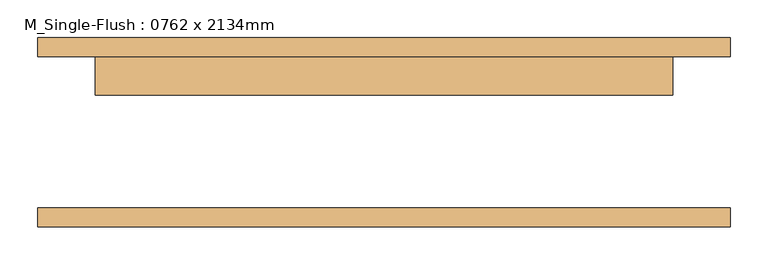
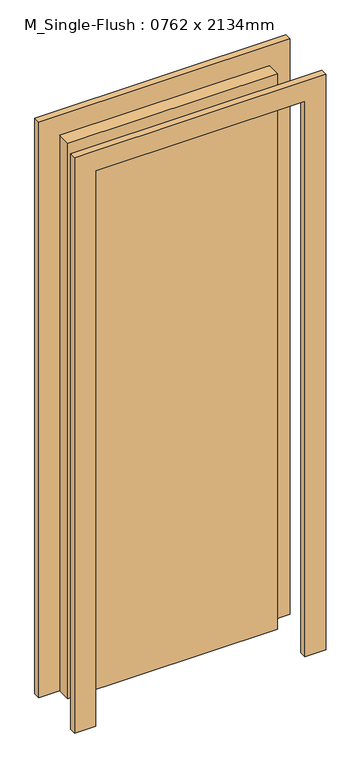
"""IFC4 building model written with IfcOpenShell, lengths in millimetres: door geometry, M_Single-Flush : 0762 x 2134mm."""

from ifc_helpers import new_model, si_unit, frame, origin, origin_with_axes, place, context, project, spatial, polyline, outline, extrude, source, transform, mapped, element, save


def m_single_flush_0762_x_2134mm_85379237(model_context):
    return source(origin(), model_context, "Body", "SweptSolid", [
        extrude(outline(polyline([(2210.0, -457.0), (0.0, -457.0), (0.0, -381.0), (2134.0, -381.0), (2134.0, 381.0), (0.0, 381.0), (0.0, 457.0), (2210.0, 457.0), (2210.0, -457.0)])), frame((0.0, 100.0, 0.0), z_axis=(0.0, 1.0, 0.0), x_axis=(0.0, 0.0, 1.0)), (0.0, 0.0, 1.0), 25.0),
        extrude(outline(polyline([(2210.0, 457.0), (2210.0, -457.0), (0.0, -457.0), (0.0, -381.0), (2134.0, -381.0), (2134.0, 381.0), (0.0, 381.0), (0.0, 457.0), (2210.0, 457.0)])), frame((0.0, -125.0, 0.0), z_axis=(0.0, 1.0, 0.0), x_axis=(0.0, 0.0, 1.0)), (0.0, 0.0, 1.0), 25.0),
        extrude(outline(polyline([(381.0, 49.0), (-381.0, 49.0), (-381.0, 100.0), (381.0, 100.0), (381.0, 49.0)])), origin_with_axes(), (0.0, 0.0, 1.0), 2134.0),
    ])


if __name__ == "__main__":
    model = new_model("IFC4")
    model_context = context("Model", 3, world=origin())
    ifc_project = project(units=[si_unit("LENGTHUNIT", "METRE", prefix="MILLI")], contexts=[model_context])
    site = spatial("IfcSite", under=ifc_project)
    building = spatial("IfcBuilding", under=site)
    placement = place(None, origin())
    m_single_flush_0762_x_2134mm_shape = m_single_flush_0762_x_2134mm_85379237(model_context)
    element("IfcDoor", 1, ObjectType="M_Single-Flush : 0762 x 2134mm", at=placement, inside=building, context=model_context, shape_type="MappedRepresentation", body=[
        mapped(m_single_flush_0762_x_2134mm_shape, transform((0.0, 0.0, 0.0), x_axis=(1.0, 0.0, 0.0), y_axis=(0.0, 1.0, 0.0), z_axis=(0.0, 0.0, 1.0))),
    ])
    save(model, "model.ifc")

# Revit data of these elements
# Type "M_Single-Flush : 0762 x 2134mm"
#   Type Mark = "18"
#   Thickness = 51 mm
#   Height = 2134 mm
#   Trim Projection Ext = 25 mm
#   Trim Projection Int = 25 mm
#   Trim Width = 76 mm
#   Width = 762 mm
#   Door Material = Door - Panel
#   Frame Material = Door - Frame
#   Function = (empty or 0)
#   Wall Closure = (empty or 0)
# Element 1 (IfcDoor, "M_Single-Flush : 0762 x 2134mm")
#   Materials on its faces: "Door - Frame", "Door - Panel"
# Materials
#   "Door - Panel": class "Wood", colour RGB 114 82 51, transparency 0
#   "Door - Frame": colour RGB 153 76 43, transparency 0
